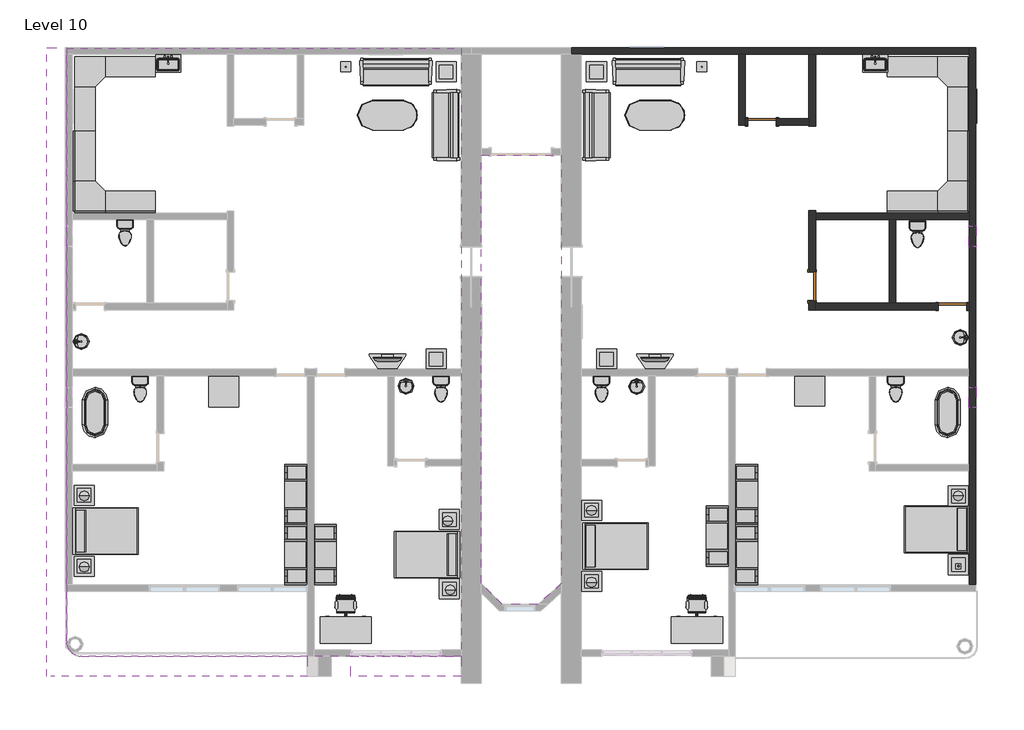
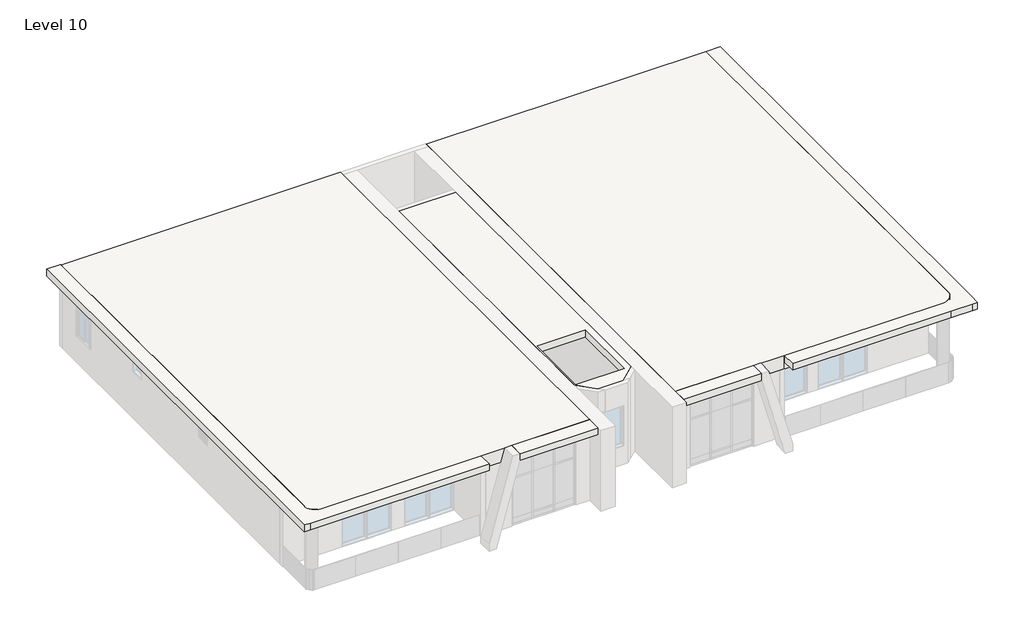
# One storey, part 3 of 3: 42 furniture elements, 14 flow terminals, 10 light fixtures, 9 walls, 4 slabs, 3 doors, 3 windows.
# Revit data of these elements (continued)
# Elements 26, 27 (IfcFurniture, "Desk : 60\" x 30\"")
#   Phase Created = New Construction
#   Materials on its faces: "Steel, Chrome Plated", "Laminate, Ivory, Matte", "Cherry"
# Elements 28, 29, 30, 31, 32, 33 (IfcFurniture, "Entertainment Center : 72\" x 72\" x 24\"")
#   Phase Created = New Construction
#   Materials on its faces: "Steel, Chrome Plated", "Glass - Clear, Grey"
# Elements 34, 35, 36, 37 (IfcFurniture, "Sofa-Pensi : 84\"")
#   Phase Created = New Construction
#   Materials on its faces: "Cherry", "Linen, Beige", "Steel, Chrome Plated"
# Elements 38, 39 (IfcFurniture, "TV - Flat Screen : 32\"")
#   Stand = yes
#   Phase Created = New Construction
#   Materials on its faces: "TV - Black", "TV - Glass", "TV - Screen"
# Elements 40, 41 (IfcFurniture, "TV Stand : TV Stand")
#   Phase Created = New Construction
#   Materials on its faces: "Melamine - Gray", "Glass - Shelves"
# Elements 42, 43, 44, 45, 46, 47, 48, 49, 50, 51, 52, 53 (IfcFurniture, "Table-Coffee : 24\" x 24\" x 24\"")
#   Phase Created = New Construction
#   Materials on its faces: "Glass - Clear, Grey"
# Elements 54, 55 (IfcFurniture, "Table-Dining Oval : 36\" x 72\"")
#   Phase Created = New Construction
#   Materials on its faces: "Steel, Chrome Plated", "Glass - Clear, Grey"
# Elements 56, 57 (IfcFurniture, "Table-Rectangular : 36\" x 36\"")
#   Phase Created = New Construction
#   Materials on its faces: "Birch"
# Elements 58, 59 (IfcFurniture, "Work Station Cubicle : 96\" x 96\"")
#   Phase Created = New Construction
#   Materials on its faces: "Textile - Light Gray", "Laminate, Ivory, Matte"
# Element 60 (IfcLightFixture, "100W - 120V")
#   Mark = "114"
#   Phase Created = New Construction
#   Materials on its faces: "Steel, Chrome Plated", "Glass, Frosted"
# Element 61 (IfcLightFixture, "100W - 120V")
#   Mark = "115"
#   Phase Created = New Construction
#   Materials on its faces: "Steel, Chrome Plated", "Glass, Frosted"
# Element 62 (IfcLightFixture, "Table Lamp - Hemispheric : 60W - 120V")
#   Mark = "116"
#   Phase Created = New Construction
#   Materials on its faces: "Steel, Chrome Plated", "Glass, Frosted", "Birch"
# Element 63 (IfcLightFixture, "Table Lamp - Hemispheric : 60W - 120V")
#   Mark = "117"
#   Phase Created = New Construction
#   Materials on its faces: "Steel, Chrome Plated", "Glass, Frosted", "Birch"
# Element 64 (IfcLightFixture, "Table Lamp - Hemispheric : 60W - 120V")
#   Mark = "118"
#   Phase Created = New Construction
#   Materials on its faces: "Steel, Chrome Plated", "Glass, Frosted", "Birch"
# Element 65 (IfcLightFixture, "Table Lamp - Hemispheric : 60W - 120V")
#   Mark = "119"
#   Phase Created = New Construction
#   Materials on its faces: "Steel, Chrome Plated", "Glass, Frosted", "Birch"
# Element 66 (IfcLightFixture, "Table Lamp - Hemispheric : 60W - 120V")
#   Mark = "120"
#   Phase Created = New Construction
#   Materials on its faces: "Steel, Chrome Plated", "Glass, Frosted", "Birch"
# Element 67 (IfcLightFixture, "Table Lamp - Hemispheric : 60W - 120V")
#   Mark = "121"
#   Phase Created = New Construction
#   Materials on its faces: "Steel, Chrome Plated", "Glass, Frosted", "Birch"
# Element 68 (IfcLightFixture, "Table Lamp - Hemispheric : 60W - 120V")
#   Mark = "122"
#   Phase Created = New Construction
#   Materials on its faces: "Steel, Chrome Plated", "Glass, Frosted", "Birch"
# Element 69 (IfcLightFixture, "Table Lamp - Hemispheric : 60W - 120V")
#   Mark = "123"
#   Phase Created = New Construction
#   Materials on its faces: "Steel, Chrome Plated", "Glass, Frosted", "Birch"
# Element 70 (IfcSlab, "Generic - 12\" cream")
#   Height Offset From Level = 12' - 0"
#   Phase Created = New Construction
#   Materials on its faces: "Parking Stripe"
# Element 71 (IfcSlab, "Generic - 12\" white")
#   built-in parameter 1001955 = 3.14159 (stored number, unit not read)
#   Height Offset From Level = 12' - 0"
#   Phase Created = New Construction
#   Materials on its faces: "Door - Frame"
# Elements 72, 73 (IfcSlab, "Generic - 12\" white")
#   Height Offset From Level = 12' - 0"
#   Phase Created = New Construction
#   Materials on its faces: "Door - Frame"
# Elements 74, 75, 76, 77, 78, 79, 80, 81 (IfcWall, "Generic - 8\" cream")
#   Top Offset = 0' - 0"
#   Base Offset = 0' - 0"
#   Unconnected Height = 10' - 0"
#   wall height = 10' - 0"
#   Phase Created = New Construction
#   Base Constraint = Level 10
#   Materials on its faces: "Parking Stripe"
# Element 82 (IfcWall, "Generic - 8\" white")
#   Top Offset = 0' - 0"
#   Base Offset = 0' - 0"
#   Unconnected Height = 10' - 0"
#   wall height = 10' - 0"
#   Phase Created = New Construction
#   Base Constraint = Level 10
#   Materials on its faces: "Door - Frame", "Parking Stripe"
# Element 83 (IfcWindow, "Louvers with Trim : 24\" x 24\"")
#   Mark = "224"
#   Phase Created = New Construction
#   Materials on its faces: "Glass", "Iron, Ductile"
# Element 84 (IfcWindow, "Louvers with Trim : 24\" x 24\"")
#   Mark = "225"
#   Phase Created = New Construction
#   Materials on its faces: "Glass", "Iron, Ductile"
# Element 85 (IfcWindow, "Slider with Trim : 36\" x 48\"")
#   Mark = "221"
#   Phase Created = New Construction
#   Materials on its faces: "Iron, Ductile", "Glass"
# Materials
#   "Wood - Birch - Solid Stained Light Low Gloss": class "Wood", colour RGB 210 159 95, transparency 0, Cost = 0
#   "Paint - Sienna": colour RGB 118 70 51, transparency 0, Cost = 0
#   "Steel, Polished": class "Metal", colour RGB 57 57 57, transparency 0, Description = "Polished steel", Cost = 0
#   "Porcelain, Linen": class "Ceramic", colour RGB 249 239 230, transparency 0, Description = "Porcelain, linen", Cost = 0
#   "Laminate, Linen, Matte": class "Plastic", colour RGB 249 239 230, transparency 0, Description = "Plastic Laminate - Linen, Matte", Cost = 0
#   "Porcelain, Ivory": class "Ceramic", colour RGB 247 247 239, transparency 0, Description = "Porcelain, ivory", Cost = 0
#   "Laminate, Ivory, Matte": class "Plastic", colour RGB 247 247 239, transparency 0, Description = "Plastic Laminate - Ivory, Matte", Cost = 0
#   "Birch": class "Wood", colour RGB 224 178 126, transparency 0, Description = "Betula Alleghaniensis", Cost = 0
#   "Linen, White": class "Textile", colour RGB 247 247 239, transparency 0, Description = "Linen, white", Cost = 0
#   "Plastic, Opaque Black": class "Plastic", colour RGB 0 0 0, transparency 0.7, Description = "Plastic, generic, opaque black", Cost = 0
#   "Textile - Slate Blue": class "Fabric", colour RGB 98 102 118, transparency 0
#   "Steel, Chrome Plated": class "Metal", colour RGB 17 17 17, transparency 0, Description = "Chromiuim plated steel", Cost = 0
#   "Cherry": class "Wood", colour RGB 226 177 128, transparency 0, Description = "Prunus Serotina", Cost = 0
#   "Linen, Beige": class "Textile", colour RGB 249 239 230, transparency 0, Description = "Linen, beige", Cost = 0
#   "Melamine - Gray": class "Wood", colour RGB 49 49 49, transparency 0
#   "Glass - Clear, Grey": class "Glass", colour RGB 252 255 255, transparency 0.64
#   "Textile - Light Gray": class "Fabric", colour RGB 204 204 204, transparency 0
#   "Glass, Frosted": class "Glass", colour RGB 250 244 225, transparency 0.55, Description = "physical material", Cost = 0
#   "Parking Stripe": class "Paint", colour RGB 250 250 91, transparency 0, Cost = 0
#   "Door - Frame": colour RGB 118 70 51, transparency 0, Cost = 0
#   "Iron, Ductile": class "Metal", colour RGB 0 0 0, transparency 0, Description = "Ductile cast iron", Cost = 0
#   "Glass": class "Glass", colour RGB 0 128 192, transparency 0.75, Description = "Soda Lime Glass", Cost = 0
#   "TV - Black": colour RGB 49 49 49, transparency 0
#   "TV - Glass": colour RGB 157 157 157, transparency 0.9
#   "TV - Screen": colour RGB 0 0 0, transparency 0
#   "Glass - Shelves": class "Glass", colour RGB 167 167 167, transparency 0.9
